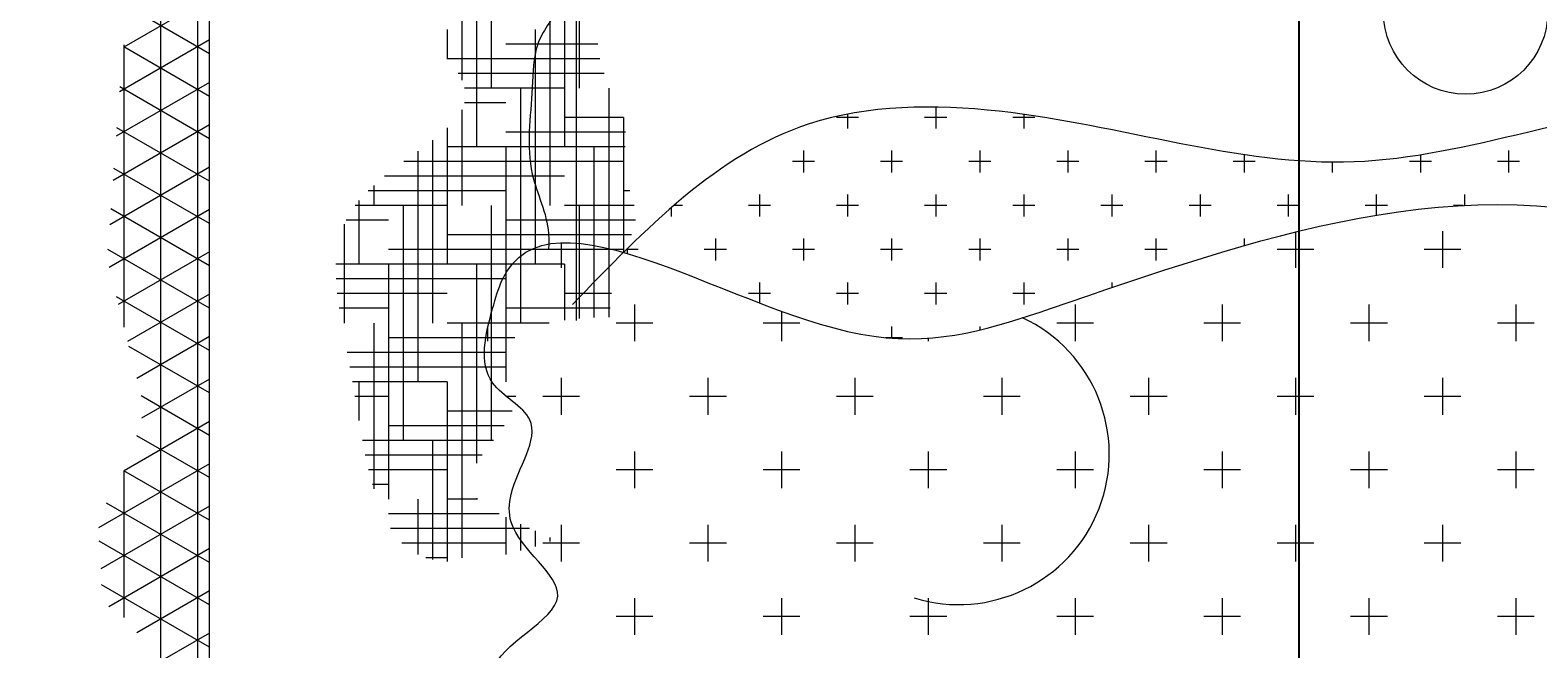
# Model space of a CAD drawing. Units: inches. Extents: x 3731 to 4318, y 1310 to 2388.
# Tile 11 of 57: x 3985 to 4038, y 1398 to 1420. Entities that reach past the tile are written whole.
import ezdxf

# ---------------------------------------------------------------- set-up
doc = ezdxf.new("R2010")
doc.units = ezdxf.units.IN
doc.layers.add('A-ANNO-DIMS', color=2, linetype='Continuous', lineweight=18)
doc.layers.add('A-FURN', color=8, linetype='Continuous', lineweight=13)
doc.styles.get("Standard").update_dxf_attribs({"font": 'arial.ttf'})
doc.dimstyles.get("Standard").update_dxf_attribs({"dimtxt": 0.18, "dimasz": 0.18, "dimexe": 0.18, "dimexo": 0.0625, "dimgap": 0.09, "dimtad": 0, "dimtih": 1, "dimtoh": 1, "dimdec": 4, "dimzin": 0, "dimdsep": 46, "dimtxsty": 'Standard', "dimcen": 0.09, "dimadec": 0, "dimazin": 0, "dimtfac": 1, "dimtdec": 4, "dimtofl": 0, "dimtmove": 0, "dimatfit": 3, "dimfxl": 1, "dimtolj": 1, "dimtzin": 0, "dimarcsym": 0})

# ---------------------------------------------------------------- blocks, each defined once
blk = doc.blocks.new('A$C200C7901')
for p, q in [((2.3121, 1.6596), (2.3121, 0.0201)), ((2, 0.2957), (2, 1.2957)), ((2.0224, 0.9977), (2.0224, 1.1977)), ((2.0224, 0.9977), (2.0224, 1.1977))]:
    blk.add_line(p, q)
at = {"linetype": 'ByBlock'}
for p, q in [((2.3224, 0.0468), (2.3224, 1.6627)), ((2.3224, 0.0468), (2.3224, 1.6627)), ((2.3537, 0.0056), (2.3537, 1.634)), ((2.3537, 0.0056), (2.3537, 1.634)), ((2.3121, 1.5619), (2.3654, 1.5926)), ((2.3121, 1.5619), (2.3654, 1.5926)), ((2.3121, 1.5738), (2.404, 1.5208)), ((2.3121, 1.5738), (2.404, 1.5208)), ((1.2004, 1.532), (1.2004, 1.5633)), ((1.2004, 1.532), (1.2004, 1.5633)), ((1.3254, 1.532), (1.3254, 1.5633)), ((1.3254, 1.532), (1.3254, 1.5633)), ((1.4504, 1.532), (1.4504, 1.5633)), ((1.4504, 1.532), (1.4504, 1.5633)), ((1.5754, 1.532), (1.5754, 1.5633)), ((1.5754, 1.532), (1.5754, 1.5633)), ((1.7004, 1.532), (1.7004, 1.5633)), ((1.7004, 1.532), (1.7004, 1.5633)), ((1.8254, 1.532), (1.8254, 1.5633)), ((1.8254, 1.532), (1.8254, 1.5633)), ((1.9504, 1.532), (1.9504, 1.5633)), ((1.9504, 1.532), (1.9504, 1.5633)), ((2.3121, 1.5258), (2.3739, 1.5615)), ((2.3121, 1.5258), (2.3739, 1.5615)), ((1.1847, 1.5477), (1.216, 1.5477)), ((1.1847, 1.5477), (1.216, 1.5477)), ((1.3097, 1.5477), (1.341, 1.5477)), ((1.3097, 1.5477), (1.341, 1.5477)), ((1.4347, 1.5477), (1.466, 1.5477)), ((1.4347, 1.5477), (1.466, 1.5477)), ((1.5597, 1.5477), (1.591, 1.5477)), ((1.5597, 1.5477), (1.591, 1.5477)), ((1.6847, 1.5477), (1.716, 1.5477)), ((1.6847, 1.5477), (1.716, 1.5477)), ((1.8097, 1.5477), (1.841, 1.5477)), ((1.8097, 1.5477), (1.841, 1.5477)), ((1.9347, 1.5477), (1.966, 1.5477)), ((1.9347, 1.5477), (1.966, 1.5477)), ((2.3849, 1.4236), (2.3849, 1.5486)), ((2.3849, 1.4236), (2.3849, 1.5486)), ((2.3121, 1.4897), (2.3979, 1.5393)), ((2.3121, 1.4897), (2.3979, 1.5393)), ((2.3121, 1.5377), (2.406, 1.4835)), ((2.3121, 1.5377), (2.406, 1.4835)), ((2.3121, 1.4537), (2.4047, 1.5071)), ((2.3121, 1.4537), (2.4047, 1.5071)), ((2.3121, 1.5016), (2.3997, 1.4511)), ((2.3121, 1.5016), (2.3997, 1.4511)), ((1.2629, 1.4695), (1.2629, 1.5008)), ((1.2629, 1.4695), (1.2629, 1.5008)), ((1.3879, 1.4695), (1.3879, 1.5008)), ((1.3879, 1.4695), (1.3879, 1.5008)), ((1.5129, 1.4695), (1.5129, 1.5008)), ((1.5129, 1.4695), (1.5129, 1.5008)), ((1.6379, 1.4695), (1.6379, 1.5008)), ((1.6379, 1.4695), (1.6379, 1.5008)), ((1.7629, 1.4695), (1.7629, 1.5008)), ((1.7629, 1.4695), (1.7629, 1.5008)), ((1.8879, 1.4695), (1.8879, 1.5008)), ((1.8879, 1.4695), (1.8879, 1.5008)), ((2.0129, 1.4695), (2.0129, 1.5008)), ((2.0129, 1.4695), (2.0129, 1.5008)), ((2.0474, 1.4691), (2.0474, 1.4915)), ((2.0474, 1.4691), (2.0474, 1.4915)), ((2.0599, 1.4631), (2.0599, 1.4948)), ((2.0599, 1.4631), (2.0599, 1.4948)), ((2.0974, 1.2977), (2.0974, 1.4977)), ((2.0974, 1.2977), (2.0974, 1.4977)), ((2.1099, 1.3477), (2.1099, 1.5009)), ((2.1099, 1.3477), (2.1099, 1.5009)), ((2.1099, 1.4977), (2.1279, 1.4977)), ((2.1099, 1.4977), (2.1279, 1.4977)), ((2.1224, 1.3977), (2.1224, 1.4992)), ((2.1224, 1.3977), (2.1224, 1.4992)), ((2.1349, 1.4477), (2.1349, 1.4949)), ((2.1349, 1.4477), (2.1349, 1.4949)), ((1.2472, 1.4852), (1.2785, 1.4852)), ((1.2472, 1.4852), (1.2785, 1.4852)), ((1.3722, 1.4852), (1.4035, 1.4852)), ((1.3722, 1.4852), (1.4035, 1.4852)), ((1.4972, 1.4852), (1.5285, 1.4852)), ((1.4972, 1.4852), (1.5285, 1.4852)), ((1.6222, 1.4852), (1.6535, 1.4852)), ((1.6222, 1.4852), (1.6535, 1.4852)), ((1.7472, 1.4852), (1.7785, 1.4852)), ((1.7472, 1.4852), (1.7785, 1.4852)), ((1.8722, 1.4852), (1.9035, 1.4852)), ((1.8722, 1.4852), (1.9035, 1.4852)), ((1.9972, 1.4852), (2.0285, 1.4852)), ((1.9972, 1.4852), (2.0285, 1.4852)), ((2.0224, 1.4805), (2.0224, 1.4839)), ((2.0224, 1.4805), (2.0224, 1.4839)), ((2.0349, 1.4748), (2.0349, 1.4879)), ((2.0349, 1.4748), (2.0349, 1.4879)), ((2.0599, 1.4852), (2.1484, 1.4852)), ((2.0599, 1.4852), (2.1484, 1.4852)), ((2.0397, 1.4727), (2.1581, 1.4727)), ((2.0397, 1.4727), (2.1581, 1.4727)), ((2.3121, 1.4176), (2.4067, 1.4721)), ((2.3121, 1.4176), (2.4067, 1.4721)), ((2.3121, 1.4655), (2.3849, 1.4235)), ((2.3121, 1.4655), (2.3849, 1.4235)), ((2.0656, 1.4602), (2.1599, 1.4602)), ((2.0656, 1.4602), (2.1599, 1.4602)), ((1.2004, 1.407), (1.2004, 1.4383)), ((1.2004, 1.407), (1.2004, 1.4383)), ((1.3254, 1.407), (1.3254, 1.4383)), ((1.3254, 1.407), (1.3254, 1.4383)), ((1.4504, 1.407), (1.4504, 1.4383)), ((1.4504, 1.407), (1.4504, 1.4383)), ((1.5754, 1.407), (1.5754, 1.4383)), ((1.5754, 1.407), (1.5754, 1.4383)), ((1.7004, 1.407), (1.7004, 1.4383)), ((1.7004, 1.407), (1.7004, 1.4383)), ((1.8254, 1.407), (1.8254, 1.4383)), ((1.8254, 1.407), (1.8254, 1.4383)), ((1.9504, 1.407), (1.9504, 1.4383)), ((1.9504, 1.407), (1.9504, 1.4383)), ((2.084, 1.4477), (2.1099, 1.4477)), ((2.084, 1.4477), (2.1099, 1.4477)), ((2.0849, 1.4468), (2.0849, 1.4477)), ((2.0849, 1.4468), (2.0849, 1.4477)), ((2.1599, 1.2477), (2.1599, 1.4477)), ((2.1599, 1.2477), (2.1599, 1.4477)), ((2.1724, 1.2977), (2.1724, 1.439)), ((2.1724, 1.2977), (2.1724, 1.439)), ((2.1599, 1.4352), (2.1735, 1.4352)), ((2.1599, 1.4352), (2.1735, 1.4352)), ((2.3121, 1.4294), (2.3741, 1.3937)), ((2.3121, 1.4294), (2.3741, 1.3937)), ((1.1847, 1.4227), (1.216, 1.4227)), ((1.1847, 1.4227), (1.216, 1.4227)), ((1.3097, 1.4227), (1.341, 1.4227)), ((1.3097, 1.4227), (1.341, 1.4227)), ((1.4347, 1.4227), (1.466, 1.4227)), ((1.4347, 1.4227), (1.466, 1.4227)), ((1.5597, 1.4227), (1.591, 1.4227)), ((1.5597, 1.4227), (1.591, 1.4227)), ((1.6847, 1.4227), (1.716, 1.4227)), ((1.6847, 1.4227), (1.716, 1.4227)), ((1.8097, 1.4227), (1.841, 1.4227)), ((1.8097, 1.4227), (1.841, 1.4227)), ((1.9347, 1.4227), (1.966, 1.4227)), ((1.9347, 1.4227), (1.966, 1.4227)), ((2.0849, 1.2477), (2.0849, 1.4171)), ((2.0849, 1.2477), (2.0849, 1.4171)), ((2.1099, 1.4227), (2.1767, 1.4227)), ((2.1099, 1.4227), (2.1767, 1.4227)), ((2.3121, 1.3815), (2.3848, 1.4235)), ((2.3121, 1.3815), (2.3848, 1.4235)), ((2.08, 1.4102), (2.1795, 1.4102)), ((2.08, 1.4102), (2.1795, 1.4102)), ((2.0703, 1.3977), (2.1819, 1.3977)), ((2.0703, 1.3977), (2.1819, 1.3977)), ((2.0724, 1.1977), (2.0724, 1.3977)), ((2.0724, 1.1977), (2.0724, 1.3977)), ((2.1474, 1.1977), (2.1474, 1.3977)), ((2.1474, 1.1977), (2.1474, 1.3977)), ((2.3121, 1.3934), (2.3703, 1.3598)), ((2.3121, 1.3934), (2.3703, 1.3598)), ((1.2629, 1.3445), (1.2629, 1.3758)), ((1.2629, 1.3445), (1.2629, 1.3758)), ((1.3879, 1.3445), (1.3879, 1.3758)), ((1.3879, 1.3445), (1.3879, 1.3758)), ((1.5129, 1.3445), (1.5129, 1.3758)), ((1.5129, 1.3445), (1.5129, 1.3758)), ((1.6379, 1.3445), (1.6379, 1.3758)), ((1.6379, 1.3445), (1.6379, 1.3758)), ((1.7629, 1.3445), (1.7629, 1.3758)), ((1.7629, 1.3445), (1.7629, 1.3758)), ((1.8879, 1.3445), (1.8879, 1.3758)), ((1.8879, 1.3445), (1.8879, 1.3758)), ((2.0129, 1.3445), (2.0129, 1.3758)), ((2.0129, 1.3445), (2.0129, 1.3758)), ((2.0612, 1.3852), (2.1599, 1.3852)), ((2.0612, 1.3852), (2.1599, 1.3852)), ((2.1849, 1.3477), (2.1849, 1.3808)), ((2.1849, 1.3477), (2.1849, 1.3808)), ((2.3121, 1.3454), (2.37, 1.3788)), ((2.3121, 1.3454), (2.37, 1.3788)), ((1.2472, 1.3602), (1.2785, 1.3602)), ((1.2472, 1.3602), (1.2785, 1.3602)), ((1.3722, 1.3602), (1.4035, 1.3602)), ((1.3722, 1.3602), (1.4035, 1.3602)), ((1.4972, 1.3602), (1.5285, 1.3602)), ((1.4972, 1.3602), (1.5285, 1.3602)), ((1.6222, 1.3602), (1.6535, 1.3602)), ((1.6222, 1.3602), (1.6535, 1.3602)), ((1.7472, 1.3602), (1.7785, 1.3602)), ((1.7472, 1.3602), (1.7785, 1.3602)), ((1.8722, 1.3602), (1.9035, 1.3602)), ((1.8722, 1.3602), (1.9035, 1.3602)), ((1.9972, 1.3602), (2.0285, 1.3602)), ((1.9972, 1.3602), (2.0285, 1.3602)), ((2.0515, 1.3602), (2.0599, 1.3602)), ((2.0515, 1.3602), (2.0599, 1.3602)), ((2.0545, 1.3727), (2.1099, 1.3727)), ((2.0545, 1.3727), (2.1099, 1.3727)), ((2.1599, 1.3602), (2.1883, 1.3602)), ((2.1599, 1.3602), (2.1883, 1.3602)), ((2.0599, 1.1477), (2.0599, 1.3477)), ((2.0599, 1.1477), (2.0599, 1.3477)), ((2.1099, 1.3477), (2.1904, 1.3477)), ((2.1099, 1.3477), (2.1904, 1.3477)), ((2.1349, 1.1515), (2.1349, 1.3477)), ((2.1349, 1.1515), (2.1349, 1.3477)), ((2.3121, 1.3573), (2.3808, 1.3176)), ((2.3121, 1.3573), (2.3808, 1.3176)), ((2.0599, 1.3352), (2.1926, 1.3352)), ((2.0599, 1.3352), (2.1926, 1.3352)), ((2.3121, 1.3093), (2.374, 1.345)), ((2.3121, 1.3093), (2.374, 1.345)), ((2.0594, 1.3227), (2.195, 1.3227)), ((2.0594, 1.3227), (2.195, 1.3227)), ((1.2004, 1.282), (1.2004, 1.3133)), ((1.2004, 1.282), (1.2004, 1.3133)), ((1.3254, 1.282), (1.3254, 1.3133)), ((1.3254, 1.282), (1.3254, 1.3133)), ((1.4504, 1.282), (1.4504, 1.3133)), ((1.4504, 1.282), (1.4504, 1.3133)), ((1.5754, 1.282), (1.5754, 1.3133)), ((1.5754, 1.282), (1.5754, 1.3133)), ((1.7004, 1.3106), (1.7004, 1.3133)), ((1.7004, 1.3106), (1.7004, 1.3133)), ((1.7222, 1.3102), (1.7369, 1.3102)), ((1.7222, 1.3102), (1.7369, 1.3102)), ((1.7316, 1.3008), (1.7316, 1.3106)), ((1.7316, 1.3008), (1.7316, 1.3106)), ((1.8254, 1.2876), (1.8254, 1.3133)), ((1.8254, 1.2876), (1.8254, 1.3133)), ((1.9504, 1.282), (1.9504, 1.3133)), ((1.9504, 1.282), (1.9504, 1.3133)), ((2.0524, 1.3102), (2.1599, 1.3102)), ((2.0524, 1.3102), (2.1599, 1.3102)), ((2.0754, 1.3017), (2.0754, 1.3133)), ((2.0754, 1.3017), (2.0754, 1.3133)), ((2.3121, 1.3212), (2.3914, 1.2754)), ((2.3121, 1.3212), (2.3914, 1.2754)), ((2.3121, 1.2732), (2.3819, 1.3135)), ((2.3121, 1.2732), (2.3819, 1.3135)), ((1.1847, 1.2977), (1.216, 1.2977)), ((1.1847, 1.2977), (1.216, 1.2977)), ((1.3097, 1.2977), (1.341, 1.2977)), ((1.3097, 1.2977), (1.341, 1.2977)), ((1.4347, 1.2977), (1.466, 1.2977)), ((1.4347, 1.2977), (1.466, 1.2977)), ((1.5597, 1.2977), (1.591, 1.2977)), ((1.5597, 1.2977), (1.591, 1.2977)), ((1.6566, 1.3008), (1.6566, 1.3036)), ((1.6566, 1.3008), (1.6566, 1.3036)), ((1.8097, 1.2977), (1.841, 1.2977)), ((1.8097, 1.2977), (1.841, 1.2977)), ((1.9347, 1.2977), (1.966, 1.2977)), ((1.9347, 1.2977), (1.966, 1.2977)), ((2.023, 1.2977), (2.1099, 1.2977)), ((2.023, 1.2977), (2.1099, 1.2977)), ((2.0474, 1.0977), (2.0474, 1.2977)), ((2.0474, 1.0977), (2.0474, 1.2977)), ((2.0597, 1.2977), (2.0744, 1.2977)), ((2.0597, 1.2977), (2.0744, 1.2977)), ((2.1224, 1.1421), (2.1224, 1.2977)), ((2.1224, 1.1421), (2.1224, 1.2977)), ((2.1974, 1.2135), (2.1974, 1.2977)), ((2.1974, 1.2135), (2.1974, 1.2977)), ((2.3849, 1.0607), (2.3849, 1.3013)), ((2.3849, 1.0607), (2.3849, 1.3013)), ((1.9711, 1.2852), (2.0599, 1.2852)), ((1.9711, 1.2852), (2.0599, 1.2852)), ((1.9724, 1.0977), (1.9724, 1.2927)), ((1.9724, 1.0977), (1.9724, 1.2927)), ((1.9849, 1.1477), (1.9849, 1.293)), ((1.9849, 1.1477), (1.9849, 1.293)), ((1.9974, 1.1977), (1.9974, 1.2939)), ((1.9974, 1.1977), (1.9974, 1.2939)), ((2.0099, 1.2477), (2.0099, 1.2953)), ((2.0099, 1.2477), (2.0099, 1.2953)), ((2.1599, 1.2852), (2.2018, 1.2852)), ((2.1599, 1.2852), (2.2018, 1.2852)), ((2.3121, 1.2851), (2.3985, 1.2352)), ((2.3121, 1.2851), (2.3985, 1.2352)), ((1.6097, 1.2727), (1.6285, 1.2727)), ((1.6097, 1.2727), (1.6285, 1.2727)), ((1.6191, 1.2633), (1.6191, 1.282)), ((1.6191, 1.2633), (1.6191, 1.282)), ((1.6847, 1.2727), (1.7035, 1.2727)), ((1.6847, 1.2727), (1.7035, 1.2727)), ((1.6941, 1.2633), (1.6941, 1.282)), ((1.6941, 1.2633), (1.6941, 1.282)), ((1.7597, 1.2727), (1.7785, 1.2727)), ((1.7597, 1.2727), (1.7785, 1.2727)), ((1.7691, 1.2633), (1.7691, 1.282)), ((1.7691, 1.2633), (1.7691, 1.282)), ((1.8347, 1.2727), (1.8535, 1.2727)), ((1.8347, 1.2727), (1.8535, 1.2727)), ((1.8441, 1.2633), (1.8441, 1.2806)), ((1.8441, 1.2633), (1.8441, 1.2806)), ((1.97, 1.2727), (2.0099, 1.2727)), ((1.97, 1.2727), (2.0099, 1.2727)), ((2.1099, 1.2727), (2.2034, 1.2727)), ((2.1099, 1.2727), (2.2034, 1.2727)), ((2.3121, 1.2371), (2.3898, 1.282)), ((2.3121, 1.2371), (2.3898, 1.282)), ((1.5441, 1.2633), (1.5441, 1.2675)), ((1.5441, 1.2633), (1.5441, 1.2675)), ((2.0599, 1.2602), (2.2044, 1.2602)), ((2.0599, 1.2602), (2.2044, 1.2602)), ((1.2629, 1.2195), (1.2629, 1.2508)), ((1.2629, 1.2195), (1.2629, 1.2508)), ((1.3879, 1.2202), (1.3879, 1.2508)), ((1.3879, 1.2202), (1.3879, 1.2508)), ((2.0099, 1.2477), (2.2045, 1.2477)), ((2.0099, 1.2477), (2.2045, 1.2477)), ((2.0129, 1.2293), (2.0129, 1.2508)), ((2.0129, 1.2293), (2.0129, 1.2508)), ((2.0349, 1.0477), (2.0349, 1.2477)), ((2.0349, 1.0477), (2.0349, 1.2477)), ((2.1099, 1.1315), (2.1099, 1.2477)), ((2.1099, 1.1315), (2.1099, 1.2477)), ((2.1849, 1.1935), (2.1849, 1.2477)), ((2.1849, 1.1935), (2.1849, 1.2477)), ((2.3121, 1.2011), (2.3976, 1.2504)), ((2.3121, 1.2011), (2.3976, 1.2504)), ((2.3121, 1.249), (2.396, 1.2006)), ((2.3121, 1.249), (2.396, 1.2006)), ((1.2472, 1.2352), (1.2785, 1.2352)), ((1.2472, 1.2352), (1.2785, 1.2352)), ((1.3722, 1.2352), (1.4035, 1.2352)), ((1.3722, 1.2352), (1.4035, 1.2352)), ((1.4316, 1.2258), (1.4316, 1.2318)), ((1.4316, 1.2258), (1.4316, 1.2318)), ((1.4972, 1.2352), (1.516, 1.2352)), ((1.4972, 1.2352), (1.516, 1.2352)), ((1.5066, 1.2258), (1.5066, 1.2445)), ((1.5066, 1.2258), (1.5066, 1.2445)), ((1.5722, 1.2352), (1.591, 1.2352)), ((1.5722, 1.2352), (1.591, 1.2352)), ((1.5816, 1.2258), (1.5816, 1.2445)), ((1.5816, 1.2258), (1.5816, 1.2445)), ((1.6472, 1.2352), (1.666, 1.2352)), ((1.6472, 1.2352), (1.666, 1.2352)), ((1.6566, 1.2258), (1.6566, 1.2445)), ((1.6566, 1.2258), (1.6566, 1.2445)), ((1.7222, 1.2352), (1.741, 1.2352)), ((1.7222, 1.2352), (1.741, 1.2352)), ((1.7316, 1.2258), (1.7316, 1.2445)), ((1.7316, 1.2258), (1.7316, 1.2445)), ((1.7972, 1.2352), (1.816, 1.2352)), ((1.7972, 1.2352), (1.816, 1.2352)), ((1.8066, 1.2258), (1.8066, 1.2445)), ((1.8066, 1.2258), (1.8066, 1.2445)), ((1.8722, 1.2352), (1.891, 1.2352)), ((1.8722, 1.2352), (1.891, 1.2352)), ((1.8816, 1.2258), (1.8816, 1.2445)), ((1.8816, 1.2258), (1.8816, 1.2445)), ((1.9472, 1.2352), (1.9574, 1.2352)), ((1.9472, 1.2352), (1.9574, 1.2352)), ((1.9566, 1.2344), (1.9566, 1.2385)), ((1.9566, 1.2344), (1.9566, 1.2385)), ((1.9599, 1.1228), (1.9599, 1.2373)), ((1.9599, 1.1228), (1.9599, 1.2373)), ((1.9599, 1.2352), (2.1599, 1.2352)), ((1.9599, 1.2352), (2.1599, 1.2352)), ((2, 1.2352), (2.0285, 1.2352)), ((2, 1.2352), (2.0285, 1.2352)), ((1.953, 1.2227), (2.1099, 1.2227)), ((1.953, 1.2227), (2.1099, 1.2227)), ((1.3941, 1.1883), (1.3941, 1.207)), ((1.3941, 1.1883), (1.3941, 1.207)), ((1.4691, 1.1883), (1.4691, 1.207)), ((1.4691, 1.1883), (1.4691, 1.207)), ((1.5441, 1.1883), (1.5441, 1.207)), ((1.5441, 1.1883), (1.5441, 1.207)), ((1.6191, 1.1883), (1.6191, 1.207)), ((1.6191, 1.1883), (1.6191, 1.207)), ((1.6941, 1.1883), (1.6941, 1.207)), ((1.6941, 1.1883), (1.6941, 1.207)), ((1.7691, 1.1883), (1.7691, 1.207)), ((1.7691, 1.1883), (1.7691, 1.207)), ((1.8441, 1.1883), (1.8441, 1.207)), ((1.8441, 1.1883), (1.8441, 1.207)), ((1.9191, 1.1995), (1.9191, 1.207)), ((1.9191, 1.1995), (1.9191, 1.207)), ((1.9495, 1.2102), (2.0599, 1.2102)), ((1.9495, 1.2102), (2.0599, 1.2102)), ((2.1599, 1.2102), (2.1959, 1.2102)), ((2.1599, 1.2102), (2.1959, 1.2102)), ((2.3121, 1.165), (2.397, 1.214)), ((2.3121, 1.165), (2.397, 1.214)), ((2.3121, 1.2129), (2.3935, 1.166)), ((2.3121, 1.2129), (2.3935, 1.166)), ((1.2441, 1.1883), (1.2441, 1.1976)), ((1.2441, 1.1883), (1.2441, 1.1976)), ((1.2452, 1.1977), (1.2535, 1.1977)), ((1.2452, 1.1977), (1.2535, 1.1977)), ((1.3097, 1.1977), (1.3285, 1.1977)), ((1.3097, 1.1977), (1.3285, 1.1977)), ((1.3191, 1.1883), (1.3191, 1.2059)), ((1.3191, 1.1883), (1.3191, 1.2059)), ((1.3847, 1.1977), (1.4035, 1.1977)), ((1.3847, 1.1977), (1.4035, 1.1977)), ((1.4597, 1.1977), (1.4785, 1.1977)), ((1.4597, 1.1977), (1.4785, 1.1977)), ((1.5347, 1.1977), (1.5535, 1.1977)), ((1.5347, 1.1977), (1.5535, 1.1977)), ((1.6097, 1.1977), (1.6285, 1.1977)), ((1.6097, 1.1977), (1.6285, 1.1977)), ((1.6847, 1.1977), (1.7035, 1.1977)), ((1.6847, 1.1977), (1.7035, 1.1977)), ((1.7597, 1.1977), (1.7785, 1.1977)), ((1.7597, 1.1977), (1.7785, 1.1977)), ((1.8347, 1.1977), (1.8535, 1.1977)), ((1.8347, 1.1977), (1.8535, 1.1977)), ((1.9097, 1.1977), (1.917, 1.1977)), ((1.9097, 1.1977), (1.917, 1.1977)), ((1.9506, 1.1977), (2.0099, 1.1977)), ((1.9506, 1.1977), (2.0099, 1.1977)), ((2.0974, 1.1161), (2.0974, 1.1977)), ((2.0974, 1.1161), (2.0974, 1.1977)), ((2.1099, 1.1977), (2.1882, 1.1977)), ((2.1099, 1.1977), (2.1882, 1.1977)), ((2.1724, 1.1807), (2.1724, 1.1977)), ((2.1724, 1.1807), (2.1724, 1.1977)), ((1.9545, 1.1852), (1.9599, 1.1852)), ((1.9545, 1.1852), (1.9599, 1.1852)), ((2.0599, 1.1852), (2.1772, 1.1852)), ((2.0599, 1.1852), (2.1772, 1.1852)), ((1.2066, 1.1508), (1.2066, 1.1695)), ((1.2066, 1.1508), (1.2066, 1.1695)), ((1.2816, 1.1547), (1.2816, 1.1695)), ((1.2816, 1.1547), (1.2816, 1.1695)), ((1.3566, 1.1608), (1.3566, 1.1695)), ((1.3566, 1.1608), (1.3566, 1.1695)), ((1.4316, 1.1544), (1.4316, 1.1695)), ((1.4316, 1.1544), (1.4316, 1.1695)), ((1.5066, 1.1508), (1.5066, 1.1695)), ((1.5066, 1.1508), (1.5066, 1.1695)), ((1.5816, 1.1508), (1.5816, 1.1695)), ((1.5816, 1.1508), (1.5816, 1.1695)), ((1.6566, 1.1508), (1.6566, 1.1695)), ((1.6566, 1.1508), (1.6566, 1.1695)), ((1.7316, 1.1508), (1.7316, 1.1695)), ((1.7316, 1.1508), (1.7316, 1.1695)), ((1.8066, 1.1508), (1.8066, 1.1695)), ((1.8066, 1.1508), (1.8066, 1.1695)), ((2.0099, 1.1727), (2.1631, 1.1727)), ((2.0099, 1.1727), (2.1631, 1.1727)), ((2.3121, 1.1768), (2.3909, 1.1314)), ((2.3121, 1.1768), (2.3909, 1.1314)), ((2.3121, 1.1289), (2.3942, 1.1763)), ((2.3121, 1.1289), (2.3942, 1.1763)), ((1.1972, 1.1602), (1.216, 1.1602)), ((1.1972, 1.1602), (1.216, 1.1602)), ((1.2722, 1.1602), (1.291, 1.1602)), ((1.2722, 1.1602), (1.291, 1.1602)), ((1.4222, 1.1602), (1.441, 1.1602)), ((1.4222, 1.1602), (1.441, 1.1602)), ((1.4972, 1.1602), (1.516, 1.1602)), ((1.4972, 1.1602), (1.516, 1.1602)), ((1.5722, 1.1602), (1.591, 1.1602)), ((1.5722, 1.1602), (1.591, 1.1602)), ((1.6472, 1.1602), (1.666, 1.1602)), ((1.6472, 1.1602), (1.666, 1.1602)), ((1.7222, 1.1602), (1.741, 1.1602)), ((1.7222, 1.1602), (1.741, 1.1602)), ((1.7972, 1.1602), (1.816, 1.1602)), ((1.7972, 1.1602), (1.816, 1.1602)), ((1.9599, 1.1602), (2.1468, 1.1602)), ((1.9599, 1.1602), (2.1468, 1.1602)), ((1.9585, 1.1477), (2.1099, 1.1477)), ((1.9585, 1.1477), (2.1099, 1.1477)), ((2.0099, 0.9477), (2.0099, 1.1477)), ((2.0099, 0.9477), (2.0099, 1.1477)), ((2.0849, 0.9477), (2.0849, 1.1477)), ((2.0849, 0.9477), (2.0849, 1.1477)), ((1.6191, 1.1201), (1.6191, 1.132)), ((1.6191, 1.1201), (1.6191, 1.132)), ((1.6941, 1.1139), (1.6941, 1.132)), ((1.6941, 1.1139), (1.6941, 1.132)), ((1.7691, 1.1198), (1.7691, 1.132)), ((1.7691, 1.1198), (1.7691, 1.132)), ((1.9581, 1.1352), (2.0599, 1.1352)), ((1.9581, 1.1352), (2.0599, 1.1352)), ((2.3121, 1.1408), (2.3884, 1.0967)), ((2.3121, 1.1408), (2.3884, 1.0967)), ((2.3121, 1.0928), (2.3915, 1.1386)), ((2.3121, 1.0928), (2.3915, 1.1386)), ((1.6097, 1.1227), (1.6285, 1.1227)), ((1.6097, 1.1227), (1.6285, 1.1227)), ((1.6847, 1.1227), (1.7035, 1.1227)), ((1.6847, 1.1227), (1.7035, 1.1227)), ((1.7597, 1.1227), (1.7785, 1.1227)), ((1.7597, 1.1227), (1.7785, 1.1227)), ((1.9599, 1.1227), (2.0099, 1.1227)), ((1.9599, 1.1227), (2.0099, 1.1227)), ((2.0599, 1.1102), (2.0951, 1.1102)), ((2.0599, 1.1102), (2.0951, 1.1102)), ((2.3121, 1.1047), (2.3851, 1.0625)), ((2.3121, 1.1047), (2.3851, 1.0625)), ((1.9974, 0.8977), (1.9974, 1.0977)), ((1.9974, 0.8977), (1.9974, 1.0977)), ((2.0099, 1.0977), (2.095, 1.0977)), ((2.0099, 1.0977), (2.095, 1.0977)), ((2.0724, 0.8977), (2.0724, 1.0977)), ((2.0724, 0.8977), (2.0724, 1.0977)), ((2.0974, 0.9977), (2.0974, 1.0909)), ((2.0974, 0.9977), (2.0974, 1.0909)), ((2.3121, 1.0567), (2.3887, 1.1009)), ((2.3121, 1.0567), (2.3887, 1.1009)), ((1.9763, 1.0852), (2.1005, 1.0852)), ((1.9763, 1.0852), (2.1005, 1.0852)), ((1.9799, 1.0727), (2.1099, 1.0727)), ((1.9799, 1.0727), (2.1099, 1.0727)), ((2.1099, 1.0477), (2.1099, 1.0729)), ((2.1099, 1.0477), (2.1099, 1.0729)), ((2.3121, 1.0686), (2.3813, 1.0286)), ((2.3121, 1.0686), (2.3813, 1.0286)), ((1.9815, 1.0602), (2.0599, 1.0602)), ((1.9815, 1.0602), (2.0599, 1.0602)), ((2.3121, 1.0206), (2.3851, 1.0628)), ((2.3121, 1.0206), (2.3851, 1.0628))]:
    blk.add_line(p, q, dxfattribs=at)
blk.add_circle((1.2431, 1.0329), 0.0699)
blk.add_arc((1.6746, 1.4093), 0.1282, 72.7909, 244.8695, dxfattribs=at)
blk.add_arc((1.6746, 1.4093), 0.1282, 72.7909, 244.8695, dxfattribs=at)
for points, knots in [([(0.4485, 1.7835), (0.4321, 1.7496), (0.4062, 1.6964), (0.49, 1.6713), (0.4719, 1.5969), (0.4123, 1.592), (0.4233, 1.5337), (0.4954, 1.5086), (0.4012, 1.4738), (0.3253, 1.4306), (0.4113, 1.3764), (0.3688, 1.3065), (0.5579, 1.2663), (0.741, 1.4533), (1.1127, 1.1109), (1.4811, 1.2478), (1.7885, 1.3492), (2.0357, 1.1637), (2.0748, 1.2974), (2.0876, 1.349), (2.0192, 1.3805), (2.0564, 1.4298), (2.0588, 1.4846), (1.9759, 1.5349), (2.1004, 1.5845), (2.0397, 1.6519), (1.971, 1.7053), (2.1104, 1.8981), (1.5946, 1.7967), (1.2448, 1.7472), (0.8129, 1.7935), (0.4953, 1.8548), (0.4582, 1.7983), (0.4485, 1.7835)], [0, 0, 0, 0, 88.420092, 139.08588, 204.302936, 239.695496, 287.801042, 327.365471, 412.960499, 463.626286, 552.059846, 584.668336, 662.614915, 940.993281, 1309.926334, 1844.022653, 1996.276242, 2316.43048, 2341.441004, 2404.707416, 2449.463774, 2514.680778, 2538.40571, 2613.031547, 2697.13096, 2760.903931, 2822.692699, 2945.47, 3215.060018, 3725.584917, 4361.974444, 4504.671998, 4555.32777, 4555.32777, 4555.32777, 4555.32777]), ([(0.4856, 1.3429), (0.5504, 1.3182), (0.6715, 1.2721), (0.8374, 1.0498), (1.1164, 1.1183), (1.3878, 1.1816), (1.5888, 1.1102), (1.8403, 1.1127), (1.9415, 1.2178), (2.0032, 1.2819)], [0, 0, 0, 0, 205.411753, 383.654933, 772.067458, 921.644661, 1226.793228, 1388.983508, 1642.292305, 1642.292305, 1642.292305, 1642.292305])]:
    blk.add_open_spline(points, degree=3, knots=knots)
blk.add_open_spline([(0.473, 1.2954), (0.4739, 1.2781), (0.4755, 1.2477), (0.5032, 1.2084), (0.4801, 1.1701), (0.4928, 1.1255), (0.4674, 1.0912), (0.4579, 1.0351), (0.501, 0.9724), (0.4311, 0.8832), (0.4902, 0.8637), (0.4843, 0.8288), (0.4774, 0.7906), (0.4625, 0.7457), (0.459, 0.6999), (0.4816, 0.6664), (0.4748, 0.625), (0.4791, 0.5889), (0.4533, 0.5528), (0.4738, 0.5004), (0.4658, 0.4502), (0.4696, 0.3946), (0.4189, 0.3935), (0.4493, 0.3684), (0.4694, 0.3857), (0.4922, 0.3576), (0.5297, 0.3262), (0.5917, 0.3353), (0.6454, 0.3754), (0.7083, 0.3741), (0.7643, 0.3328), (0.826, 0.346), (0.925, 0.3388), (1.0353, 0.3593), (1.1561, 0.3744), (1.2477, 0.3154), (1.3302, 0.3474), (1.4086, 0.3512), (1.5217, 0.3878), (1.6362, 0.3176), (1.7682, 0.3285), (1.8402, 0.3019), (1.9071, 0.3529), (1.9647, 0.3412), (2.0795, 0.2948), (2.0472, 0.3498), (2.0343, 0.3772), (2.0435, 0.43), (2.0109, 0.5782), (2.0746, 0.4643), (2.0805, 0.584), (2.0084, 0.5979), (2.0343, 0.6846), (2.0344, 0.746), (2.0293, 0.8096), (2.0489, 0.8545), (2.0652, 0.9218), (1.9842, 0.9297), (2.0007, 1.0162), (2.0367, 1.0585), (2.0367, 1.1102), (2.0457, 1.1647), (2.0226, 1.2084), (2.0234, 1.2306), (2.0236, 1.2352)], degree=3, knots=[0, 0, 0, 0, 51.660678, 90.967412, 128.902454, 170.303599, 219.852997, 247.834962, 336.321557, 429.35469, 458.821847, 477.222321, 524.135809, 581.038434, 617.839381, 657.146115, 693.947125, 740.178081, 760.753248, 820.731705, 885.133458, 928.777044, 953.563729, 976.574207, 995.553042, 1018.563482, 1064.584401, 1147.951297, 1174.787598, 1266.851571, 1308.018447, 1377.066427, 1441.511314, 1608.245014, 1714.11869, 1792.771707, 1913.247991, 1954.931389, 2029.864445, 2259.189419, 2305.221512, 2429.507982, 2456.344283, 2543.92595, 2627.925037, 2662.96218, 2687.736879, 2719.937755, 2839.540991, 2875.47895, 2953.681041, 2993.270313, 3066.872333, 3154.395764, 3200.397042, 3248.426375, 3312.828127, 3347.881398, 3444.484026, 3481.577522, 3518.665244, 3592.267265, 3644.719162, 3658.519501, 3658.519501, 3658.519501, 3658.519501], dxfattribs=at)
blk = doc.blocks.new('*D32')
at = {"layer": 'A-ANNO-DIMS', "color": 0, "lineweight": -2, "transparency": 16777216}
for p, q in [((4269.211, 1592.319), (4269.211, 1310.251)), ((3835.209, 1359.319), (3835.209, 1310.251)), ((3835.389, 1310.431), (4051.918, 1310.431)), ((4269.031, 1310.431), (4052.502, 1310.431))]:
    blk.add_line(p, q, dxfattribs=at)
at = {"layer": 'A-ANNO-DIMS', "color": 0, "transparency": 16777216}
for points in [[(3835.389, 1310.461), (3835.389, 1310.401), (3835.209, 1310.431)], [(4269.031, 1310.461), (4269.031, 1310.401), (4269.211, 1310.431)]]:
    blk.add_solid(points, dxfattribs=at)
at = {"layer": 'Defpoints', "color": 0, "transparency": 16777216}
for p in [(4269.211, 1592.382), (3835.209, 1359.382), (4269.211, 1310.431)]:
    blk.add_point(p, dxfattribs=at)
at = {"layer": 'A-ANNO-DIMS', "color": 0, "transparency": 16777216, "insert": (4052.21, 1310.431), "char_height": 0.18, "attachment_point": 5}
blk.add_mtext('\\A1;434', dxfattribs=at)
blk = doc.blocks.new('*D44')
at = {"layer": 'A-ANNO-DIMS', "color": 0, "lineweight": -2, "transparency": 16777216}
for p, q in [((3969.209, 1874.319), (3969.209, 1310.251)), ((4029.209, 1874.319), (4029.209, 1310.251)), ((3969.389, 1310.431), (3998.99, 1310.431)), ((4029.029, 1310.431), (3999.428, 1310.431))]:
    blk.add_line(p, q, dxfattribs=at)
at = {"layer": 'A-ANNO-DIMS', "color": 0, "transparency": 16777216}
for points in [[(3969.389, 1310.461), (3969.389, 1310.401), (3969.209, 1310.431)], [(4029.029, 1310.461), (4029.029, 1310.401), (4029.209, 1310.431)]]:
    blk.add_solid(points, dxfattribs=at)
at = {"layer": 'Defpoints', "color": 0, "transparency": 16777216}
for p in [(3969.209, 1874.382), (4029.209, 1874.382), (4029.209, 1310.431)]:
    blk.add_point(p, dxfattribs=at)
at = {"layer": 'A-ANNO-DIMS', "color": 0, "transparency": 16777216, "insert": (3999.209, 1310.431), "char_height": 0.18, "attachment_point": 5}
blk.add_mtext('\\A1;60', dxfattribs=at)

msp = doc.modelspace()

# ---------------------------------------------------------------- block references
at = {"layer": 'A-FURN', "xscale": 41.1071563136412, "yscale": 41.1071563136412, "zscale": 41.1071563136412, "rotation": 180}
msp.add_blockref('A$C200C7901', (4086.148, 1463.037), dxfattribs=at)

# ---------------------------------------------------------------- dimensions: what is measured, and where the dimension line sits
at = {"layer": 'A-ANNO-DIMS'}
for base, p1, p2, picture, middle in [((4029.209, 1310.431), (3969.209, 1874.382), (4029.209, 1874.382), '*D44', (3999.209, 1310.431)), ((4269.211, 1310.431), (3835.209, 1359.382), (4269.211, 1592.382), '*D32', (4052.21, 1310.431))]:
    dim = msp.add_linear_dim(base=base, p1=p1, p2=p2, dimstyle='Standard', override={"dimdec": 0, "dimlfac": 1, "dimrnd": 0, "dimzin": 0, "dimdsep": 46, "dimlunit": 2}, dxfattribs=at)
    dim.commit()
    dim.dimension.update_dxf_attribs({"geometry": picture, "text_midpoint": middle})

doc.saveas('drawing.dxf')
